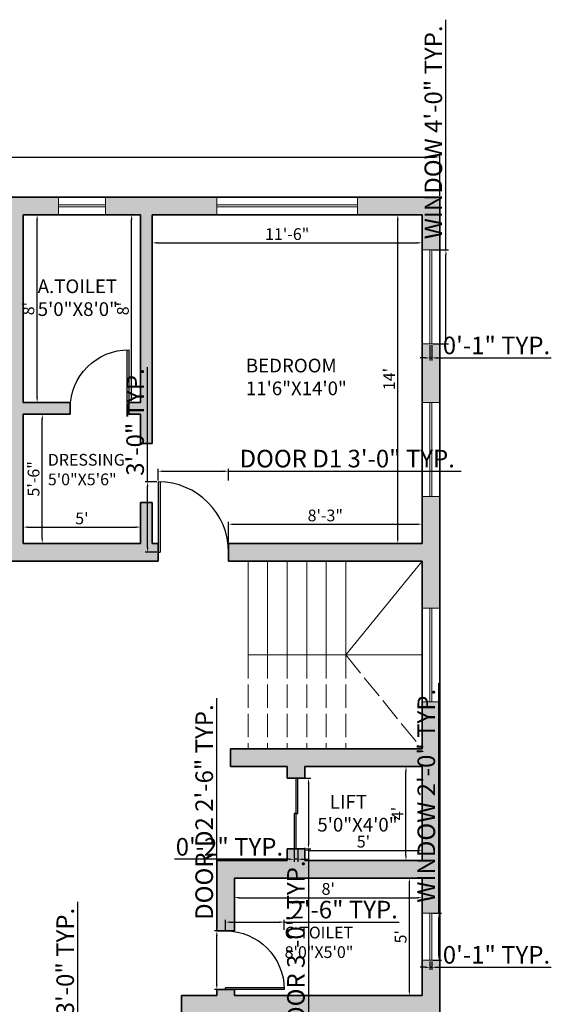
# Model space of a CAD drawing. Units: inches. Extents: x 4606 to 5879, y 1332 to 2209.
# Tile 7 of 7: x 5607 to 5879, y 1669 to 2172. Entities that reach past the tile are written whole.
import ezdxf

# ---------------------------------------------------------------- set-up
doc = ezdxf.new("R2010")
doc.units = ezdxf.units.IN
doc.linetypes.add('ACAD_ISO02W100', pattern=[15, 12, -3])
for name, color, linetype, lineweight in [('A-ANNO-DIMS', 2, 'Continuous', 18), ('A-AREA-IDEN', 7, 'Continuous', 18), ('A-DOOR', 4, 'Continuous', 25), ('A-FLOR-STRS', 7, 'Continuous', 20), ('A-FLOR-STRS-OVHD', 8, 'ACAD_ISO02W100', 13), ('A-WALL', 7, 'Continuous', 35), ('A-WALL-PATT', 252, 'Continuous', 13), ('window', 130, 'Continuous', 18)]:
    doc.layers.add(name, color=color, linetype=linetype, lineweight=lineweight)
doc.styles.get("Standard").update_dxf_attribs({"font": 'arial.ttf'})
doc.dimstyles.new('ISO-25', dxfattribs={"dimtxt": 9, "dimasz": 2.5, "dimexe": 1.25, "dimexo": 0.625, "dimtad": 1, "dimlunit": 3, "dimtxsty": 'Standard', "dimcen": 2.5, "dimadec": 0, "dimazin": 0, "dimtfac": 1, "dimtmove": 0, "dimatfit": 3, "dimfxl": 1, "dimarcsym": 0})

# ---------------------------------------------------------------- blocks, each defined once
blk = doc.blocks.new('*D25')
at = {"layer": 'A-ANNO-DIMS', "color": 0, "lineweight": -2, "transparency": 16777216}
for p, q in [((5344.86, 2081.86), (5344.86, 2102.96)), ((5347.36, 2101.71), (5819.36, 2101.71)), ((5821.86, 2081.86), (5821.86, 2102.96))]:
    blk.add_line(p, q, dxfattribs=at)
at = {"layer": 'A-ANNO-DIMS', "color": 0, "transparency": 16777216}
for points in [[(5347.36, 2102.13), (5347.36, 2101.29), (5344.86, 2101.71)], [(5819.36, 2102.13), (5819.36, 2101.29), (5821.86, 2101.71)]]:
    blk.add_solid(points, dxfattribs=at)
at = {"layer": 'Defpoints', "color": 0, "transparency": 16777216}
for p in [(5821.86, 2101.71), (5344.86, 2081.24), (5821.86, 2081.24)]:
    blk.add_point(p, dxfattribs=at)
at = {"layer": 'A-ANNO-DIMS', "color": 0, "transparency": 16777216, "insert": (5583.36, 2106.93), "char_height": 9, "attachment_point": 5}
blk.add_mtext('39\'-9"', dxfattribs=at)
blk = doc.blocks.new('D1')
for p, q in [((0, 36), (0, 0)), ((1, 36), (1, 0)), ((0, 0), (1, 0))]:
    blk.add_line(p, q)
blk.add_arc((0, 0), 36, 0, 90)
blk = doc.blocks.new('D2')
for p, q in [((0, 30), (0, 0)), ((1, 30), (1, 0)), ((0, 0), (1, 0))]:
    blk.add_line(p, q)
blk.add_arc((0, 0), 30, 0, 90)
blk = doc.blocks.new('*D29')
at = {"layer": 'A-ANNO-DIMS', "color": 0, "lineweight": -2, "transparency": 16777216}
for p, q in [((5674.86, 2071.61), (5674.86, 2056.59)), ((5812.86, 2071.61), (5812.86, 2056.59)), ((5677.36, 2057.84), (5810.36, 2057.84))]:
    blk.add_line(p, q, dxfattribs=at)
at = {"layer": 'A-ANNO-DIMS', "color": 0, "transparency": 16777216}
for points in [[(5677.36, 2058.26), (5677.36, 2057.43), (5674.86, 2057.84)], [(5810.36, 2058.26), (5810.36, 2057.43), (5812.86, 2057.84)]]:
    blk.add_solid(points, dxfattribs=at)
at = {"layer": 'Defpoints', "color": 0, "transparency": 16777216}
for p in [(5674.86, 2072.24), (5812.86, 2072.24), (5812.86, 2057.84)]:
    blk.add_point(p, dxfattribs=at)
at = {"layer": 'A-ANNO-DIMS', "color": 0, "transparency": 16777216, "insert": (5743.86, 2061.53), "char_height": 6, "attachment_point": 5}
blk.add_mtext('11\'-6"', dxfattribs=at)
blk = doc.blocks.new('*D30')
at = {"layer": 'A-ANNO-DIMS', "color": 0, "lineweight": -2, "transparency": 16777216}
for p, q in [((5812.24, 2072.24), (5799.17, 2072.24)), ((5800.42, 1906.74), (5800.42, 2069.74)), ((5812.24, 1904.24), (5799.17, 1904.24))]:
    blk.add_line(p, q, dxfattribs=at)
at = {"layer": 'A-ANNO-DIMS', "color": 0, "transparency": 16777216}
for points in [[(5800.01, 2069.74), (5800.84, 2069.74), (5800.42, 2072.24)], [(5800.01, 1906.74), (5800.84, 1906.74), (5800.42, 1904.24)]]:
    blk.add_solid(points, dxfattribs=at)
at = {"layer": 'Defpoints', "color": 0, "transparency": 16777216}
for p in [(5800.42, 2072.24), (5812.86, 2072.24), (5812.86, 1904.24)]:
    blk.add_point(p, dxfattribs=at)
at = {"layer": 'A-ANNO-DIMS', "color": 0, "transparency": 16777216, "insert": (5796.79, 1988.24), "char_height": 6, "attachment_point": 5, "rotation": 90}
blk.add_mtext("14'", dxfattribs=at)
blk = doc.blocks.new('*D33')
at = {"layer": 'A-ANNO-DIMS', "color": 0, "lineweight": -2, "transparency": 16777216}
for p, q in [((5609.49, 2072.24), (5617.21, 2072.24)), ((5615.96, 1978.74), (5615.96, 2069.74)), ((5609.49, 1976.24), (5617.21, 1976.24))]:
    blk.add_line(p, q, dxfattribs=at)
at = {"layer": 'A-ANNO-DIMS', "color": 0, "transparency": 16777216}
for points in [[(5615.54, 2069.74), (5616.37, 2069.74), (5615.96, 2072.24)], [(5615.54, 1978.74), (5616.37, 1978.74), (5615.96, 1976.24)]]:
    blk.add_solid(points, dxfattribs=at)
at = {"layer": 'Defpoints', "color": 0, "transparency": 16777216}
for p in [(5608.86, 2072.24), (5615.96, 2072.24), (5608.86, 1976.24)]:
    blk.add_point(p, dxfattribs=at)
at = {"layer": 'A-ANNO-DIMS', "color": 0, "transparency": 16777216, "insert": (5612.27, 2024.24), "char_height": 6, "attachment_point": 5, "rotation": 90}
blk.add_mtext("8'", dxfattribs=at)
blk = doc.blocks.new('*D34')
at = {"layer": 'A-ANNO-DIMS', "color": 0, "lineweight": -2, "transparency": 16777216}
for p, q in [((5668.24, 2072.24), (5663.04, 2072.24)), ((5664.29, 1978.74), (5664.29, 2069.74)), ((5668.24, 1976.24), (5663.04, 1976.24))]:
    blk.add_line(p, q, dxfattribs=at)
at = {"layer": 'A-ANNO-DIMS', "color": 0, "transparency": 16777216}
for points in [[(5663.87, 2069.74), (5664.71, 2069.74), (5664.29, 2072.24)], [(5663.87, 1978.74), (5664.71, 1978.74), (5664.29, 1976.24)]]:
    blk.add_solid(points, dxfattribs=at)
at = {"layer": 'Defpoints', "color": 0, "transparency": 16777216}
for p in [(5664.29, 2072.24), (5668.86, 2072.24), (5668.86, 1976.24)]:
    blk.add_point(p, dxfattribs=at)
at = {"layer": 'A-ANNO-DIMS', "color": 0, "transparency": 16777216, "insert": (5660.6, 2024.24), "char_height": 6, "attachment_point": 5, "rotation": 90}
blk.add_mtext("8'", dxfattribs=at)
blk = doc.blocks.new('*D39')
at = {"layer": 'A-ANNO-DIMS', "color": 0, "lineweight": -2, "transparency": 16777216}
for p, q in [((5609.49, 1970.24), (5619.83, 1970.24)), ((5618.58, 1906.74), (5618.58, 1967.74)), ((5609.49, 1904.24), (5619.83, 1904.24))]:
    blk.add_line(p, q, dxfattribs=at)
at = {"layer": 'A-ANNO-DIMS', "color": 0, "transparency": 16777216}
for points in [[(5618.17, 1967.74), (5619, 1967.74), (5618.58, 1970.24)], [(5618.17, 1906.74), (5619, 1906.74), (5618.58, 1904.24)]]:
    blk.add_solid(points, dxfattribs=at)
at = {"layer": 'Defpoints', "color": 0, "transparency": 16777216}
for p in [(5608.86, 1970.24), (5618.58, 1970.24), (5608.86, 1904.24)]:
    blk.add_point(p, dxfattribs=at)
at = {"layer": 'A-ANNO-DIMS', "color": 0, "transparency": 16777216, "insert": (5614.89, 1937.24), "char_height": 6, "attachment_point": 5, "rotation": 90}
blk.add_mtext('5\'-6"', dxfattribs=at)
blk = doc.blocks.new('*D40')
at = {"layer": 'A-ANNO-DIMS', "color": 0, "lineweight": -2, "transparency": 16777216}
for p, q in [((5608.86, 1904.86), (5608.86, 1913.83)), ((5611.36, 1912.58), (5666.36, 1912.58)), ((5668.86, 1904.86), (5668.86, 1913.83))]:
    blk.add_line(p, q, dxfattribs=at)
at = {"layer": 'A-ANNO-DIMS', "color": 0, "transparency": 16777216}
for points in [[(5611.36, 1913), (5611.36, 1912.16), (5608.86, 1912.58)], [(5666.36, 1913), (5666.36, 1912.16), (5668.86, 1912.58)]]:
    blk.add_solid(points, dxfattribs=at)
at = {"layer": 'Defpoints', "color": 0, "transparency": 16777216}
for p in [(5668.86, 1912.58), (5608.86, 1904.24), (5668.86, 1904.24)]:
    blk.add_point(p, dxfattribs=at)
at = {"layer": 'A-ANNO-DIMS', "color": 0, "transparency": 16777216, "insert": (5638.86, 1916.26), "char_height": 6, "attachment_point": 5}
blk.add_mtext("5'", dxfattribs=at)
blk = doc.blocks.new('*D41')
at = {"layer": 'A-ANNO-DIMS', "color": 0, "lineweight": -2, "transparency": 16777216}
for p, q in [((5713.86, 1904.86), (5713.86, 1915.32)), ((5716.36, 1914.07), (5810.36, 1914.07)), ((5812.86, 1904.86), (5812.86, 1915.32))]:
    blk.add_line(p, q, dxfattribs=at)
at = {"layer": 'A-ANNO-DIMS', "color": 0, "transparency": 16777216}
for points in [[(5716.36, 1914.48), (5716.36, 1913.65), (5713.86, 1914.07)], [(5810.36, 1914.48), (5810.36, 1913.65), (5812.86, 1914.07)]]:
    blk.add_solid(points, dxfattribs=at)
at = {"layer": 'Defpoints', "color": 0, "transparency": 16777216}
for p in [(5812.86, 1914.07), (5713.86, 1904.24), (5812.86, 1904.24)]:
    blk.add_point(p, dxfattribs=at)
at = {"layer": 'A-ANNO-DIMS', "color": 0, "transparency": 16777216, "insert": (5763.36, 1917.76), "char_height": 6, "attachment_point": 5}
blk.add_mtext('8\'-3"', dxfattribs=at)
blk = doc.blocks.new('*D49')
at = {"layer": 'A-ANNO-DIMS', "color": 0, "lineweight": -2, "transparency": 16777216}
for p, q in [((5812.24, 1733.24), (5805.1, 1733.24)), ((5806.35, 1675.74), (5806.35, 1730.74)), ((5812.24, 1673.24), (5805.1, 1673.24))]:
    blk.add_line(p, q, dxfattribs=at)
at = {"layer": 'A-ANNO-DIMS', "color": 0, "transparency": 16777216}
for points in [[(5805.94, 1730.74), (5806.77, 1730.74), (5806.35, 1733.24)], [(5805.94, 1675.74), (5806.77, 1675.74), (5806.35, 1673.24)]]:
    blk.add_solid(points, dxfattribs=at)
at = {"layer": 'Defpoints', "color": 0, "transparency": 16777216}
for p in [(5806.35, 1733.24), (5812.86, 1733.24), (5812.86, 1673.24)]:
    blk.add_point(p, dxfattribs=at)
at = {"layer": 'A-ANNO-DIMS', "color": 0, "transparency": 16777216, "insert": (5802.68, 1703.24), "char_height": 6, "attachment_point": 5, "rotation": 90}
blk.add_mtext("5'", dxfattribs=at)
blk = doc.blocks.new('*D50')
at = {"layer": 'A-ANNO-DIMS', "color": 0, "lineweight": -2, "transparency": 16777216}
for p, q in [((5716.86, 1732.61), (5716.86, 1721.98)), ((5812.86, 1732.61), (5812.86, 1721.98)), ((5719.36, 1723.23), (5810.36, 1723.23))]:
    blk.add_line(p, q, dxfattribs=at)
at = {"layer": 'A-ANNO-DIMS', "color": 0, "transparency": 16777216}
for points in [[(5719.36, 1723.65), (5719.36, 1722.82), (5716.86, 1723.23)], [(5810.36, 1723.65), (5810.36, 1722.82), (5812.86, 1723.23)]]:
    blk.add_solid(points, dxfattribs=at)
at = {"layer": 'Defpoints', "color": 0, "transparency": 16777216}
for p in [(5716.86, 1733.24), (5812.86, 1733.24), (5812.86, 1723.23)]:
    blk.add_point(p, dxfattribs=at)
at = {"layer": 'A-ANNO-DIMS', "color": 0, "transparency": 16777216, "insert": (5764.86, 1726.92), "char_height": 6, "attachment_point": 5}
blk.add_mtext("8'", dxfattribs=at)
blk = doc.blocks.new('*D51')
at = {"layer": 'A-ANNO-DIMS', "color": 0, "lineweight": -2, "transparency": 16777216}
for p, q in [((5752.86, 1742.86), (5752.86, 1748.66)), ((5755.36, 1747.41), (5810.36, 1747.41)), ((5812.86, 1742.86), (5812.86, 1748.66))]:
    blk.add_line(p, q, dxfattribs=at)
at = {"layer": 'A-ANNO-DIMS', "color": 0, "transparency": 16777216}
for points in [[(5755.36, 1747.82), (5755.36, 1746.99), (5752.86, 1747.41)], [(5810.36, 1747.82), (5810.36, 1746.99), (5812.86, 1747.41)]]:
    blk.add_solid(points, dxfattribs=at)
at = {"layer": 'Defpoints', "color": 0, "transparency": 16777216}
for p in [(5812.86, 1747.41), (5752.86, 1742.24), (5812.86, 1742.24)]:
    blk.add_point(p, dxfattribs=at)
at = {"layer": 'A-ANNO-DIMS', "color": 0, "transparency": 16777216, "insert": (5782.86, 1751.08), "char_height": 6, "attachment_point": 5}
blk.add_mtext("5'", dxfattribs=at)
blk = doc.blocks.new('*D52')
at = {"layer": 'A-ANNO-DIMS', "color": 0, "lineweight": -2, "transparency": 16777216}
for p, q in [((5812.24, 1790.24), (5803.37, 1790.24)), ((5804.62, 1744.74), (5804.62, 1787.74)), ((5812.24, 1742.24), (5803.37, 1742.24))]:
    blk.add_line(p, q, dxfattribs=at)
at = {"layer": 'A-ANNO-DIMS', "color": 0, "transparency": 16777216}
for points in [[(5804.21, 1787.74), (5805.04, 1787.74), (5804.62, 1790.24)], [(5804.21, 1744.74), (5805.04, 1744.74), (5804.62, 1742.24)]]:
    blk.add_solid(points, dxfattribs=at)
at = {"layer": 'Defpoints', "color": 0, "transparency": 16777216}
for p in [(5804.62, 1790.24), (5812.86, 1790.24), (5812.86, 1742.24)]:
    blk.add_point(p, dxfattribs=at)
at = {"layer": 'A-ANNO-DIMS', "color": 0, "transparency": 16777216, "insert": (5801, 1766.24), "char_height": 6, "attachment_point": 5, "rotation": 90}
blk.add_mtext("4'", dxfattribs=at)
blk = doc.blocks.new('GLAZING-72IN')
for p, q in [((0, 0), (0, 72)), ((1, 0), (1, 72))]:
    blk.add_line(p, q)
blk = doc.blocks.new('GLAZING-24IN')
for p, q in [((0, 0), (0, 24)), ((1, 0), (1, 24))]:
    blk.add_line(p, q)
blk = doc.blocks.new('GLAZING-48IN')
for p, q in [((0, 0), (0, 48)), ((1, 0), (1, 48))]:
    blk.add_line(p, q)
blk = doc.blocks.new('LIFT-DOOR-36IN')
for p, q in [((1, 0), (1, 36)), ((2, 18), (2, 36)), ((1, 18), (0, 18)), ((0, 18), (0, 0)), ((1, 18), (2, 18))]:
    blk.add_line(p, q)
blk = doc.blocks.new('*D67')
at = {"layer": 'A-ANNO-DIMS', "color": 0, "lineweight": -2, "transparency": 16777216}
for p, q in [((5825.06, 2054.24), (5825.06, 2171.88)), ((5818.49, 2054.24), (5826.31, 2054.24)), ((5825.06, 2008.74), (5825.06, 2051.74)), ((5818.49, 2006.24), (5826.31, 2006.24))]:
    blk.add_line(p, q, dxfattribs=at)
at = {"layer": 'A-ANNO-DIMS', "color": 0, "transparency": 16777216}
for points in [[(5824.65, 2051.74), (5825.48, 2051.74), (5825.06, 2054.24)], [(5824.65, 2008.74), (5825.48, 2008.74), (5825.06, 2006.24)]]:
    blk.add_solid(points, dxfattribs=at)
at = {"layer": 'Defpoints', "color": 0, "transparency": 16777216}
for p in [(5817.86, 2054.24), (5825.06, 2054.24), (5817.86, 2006.24)]:
    blk.add_point(p, dxfattribs=at)
at = {"layer": 'A-ANNO-DIMS', "color": 0, "transparency": 16777216, "insert": (5819.78, 2114.31), "char_height": 9, "attachment_point": 5, "rotation": 90}
blk.add_mtext('WINDOW 4\'-0" TYP.', dxfattribs=at)
blk = doc.blocks.new('*D68')
at = {"layer": 'A-ANNO-DIMS', "color": 0, "lineweight": -2, "transparency": 16777216}
for p, q in [((5816.86, 2005.61), (5816.86, 1997.79)), ((5817.86, 2005.61), (5817.86, 1997.79)), ((5814.36, 1999.04), (5811.86, 1999.04)), ((5816.86, 1999.04), (5817.86, 1999.04)), ((5820.36, 1999.04), (5878.97, 1999.04))]:
    blk.add_line(p, q, dxfattribs=at)
at = {"layer": 'A-ANNO-DIMS', "color": 0, "transparency": 16777216}
for points in [[(5814.36, 1999.46), (5814.36, 1998.62), (5816.86, 1999.04)], [(5820.36, 1999.46), (5820.36, 1998.62), (5817.86, 1999.04)]]:
    blk.add_solid(points, dxfattribs=at)
at = {"layer": 'Defpoints', "color": 0, "transparency": 16777216}
for p in [(5816.86, 2006.24), (5817.86, 2006.24), (5817.86, 1999.04)]:
    blk.add_point(p, dxfattribs=at)
at = {"layer": 'A-ANNO-DIMS', "color": 0, "transparency": 16777216, "insert": (5850.92, 2004.26), "char_height": 9, "attachment_point": 5}
blk.add_mtext('0\'-1" TYP.', dxfattribs=at)
blk = doc.blocks.new('*D71')
at = {"layer": 'A-ANNO-DIMS', "color": 0, "lineweight": -2, "transparency": 16777216}
for p, q in [((5821.46, 1715.24), (5821.46, 1832.88)), ((5818.49, 1715.24), (5822.71, 1715.24)), ((5821.46, 1693.74), (5821.46, 1712.74)), ((5818.49, 1691.24), (5822.71, 1691.24))]:
    blk.add_line(p, q, dxfattribs=at)
at = {"layer": 'A-ANNO-DIMS', "color": 0, "transparency": 16777216}
for points in [[(5821.05, 1712.74), (5821.88, 1712.74), (5821.46, 1715.24)], [(5821.05, 1693.74), (5821.88, 1693.74), (5821.46, 1691.24)]]:
    blk.add_solid(points, dxfattribs=at)
at = {"layer": 'Defpoints', "color": 0, "transparency": 16777216}
for p in [(5817.86, 1715.24), (5821.46, 1715.24), (5817.86, 1691.24)]:
    blk.add_point(p, dxfattribs=at)
at = {"layer": 'A-ANNO-DIMS', "color": 0, "transparency": 16777216, "insert": (5816.18, 1775.31), "char_height": 9, "attachment_point": 5, "rotation": 90}
blk.add_mtext('WINDOW 2\'-0" TYP.', dxfattribs=at)
blk = doc.blocks.new('*D72')
at = {"layer": 'A-ANNO-DIMS', "color": 0, "lineweight": -2, "transparency": 16777216}
for p, q in [((5816.86, 1690.61), (5816.86, 1686.39)), ((5817.86, 1690.61), (5817.86, 1686.39)), ((5814.36, 1687.64), (5811.86, 1687.64)), ((5816.86, 1687.64), (5817.86, 1687.64)), ((5820.36, 1687.64), (5878.97, 1687.64))]:
    blk.add_line(p, q, dxfattribs=at)
at = {"layer": 'A-ANNO-DIMS', "color": 0, "transparency": 16777216}
for points in [[(5814.36, 1688.06), (5814.36, 1687.22), (5816.86, 1687.64)], [(5820.36, 1688.06), (5820.36, 1687.22), (5817.86, 1687.64)]]:
    blk.add_solid(points, dxfattribs=at)
at = {"layer": 'Defpoints', "color": 0, "transparency": 16777216}
for p in [(5816.86, 1691.24), (5817.86, 1691.24), (5817.86, 1687.64)]:
    blk.add_point(p, dxfattribs=at)
at = {"layer": 'A-ANNO-DIMS', "color": 0, "transparency": 16777216, "insert": (5850.92, 1692.86), "char_height": 9, "attachment_point": 5}
blk.add_mtext('0\'-1" TYP.', dxfattribs=at)
blk = doc.blocks.new('*D73')
at = {"layer": 'A-ANNO-DIMS', "color": 0, "lineweight": -2, "transparency": 16777216}
for p, q in [((5707.86, 1706.24), (5707.86, 1825.18)), ((5711.74, 1706.24), (5706.61, 1706.24)), ((5707.86, 1678.74), (5707.86, 1703.74)), ((5711.74, 1676.24), (5706.61, 1676.24))]:
    blk.add_line(p, q, dxfattribs=at)
at = {"layer": 'A-ANNO-DIMS', "color": 0, "transparency": 16777216}
for points in [[(5707.45, 1703.74), (5708.28, 1703.74), (5707.86, 1706.24)], [(5707.45, 1678.74), (5708.28, 1678.74), (5707.86, 1676.24)]]:
    blk.add_solid(points, dxfattribs=at)
at = {"layer": 'Defpoints', "color": 0, "transparency": 16777216}
for p in [(5707.86, 1706.24), (5712.36, 1706.24), (5712.36, 1676.24)]:
    blk.add_point(p, dxfattribs=at)
at = {"layer": 'A-ANNO-DIMS', "color": 0, "transparency": 16777216, "insert": (5702.58, 1766.96), "char_height": 9, "attachment_point": 5, "rotation": 90}
blk.add_mtext('DOOR D2 2\'-6" TYP.', dxfattribs=at)
blk = doc.blocks.new('*D74')
at = {"layer": 'A-ANNO-DIMS', "color": 0, "lineweight": -2, "transparency": 16777216}
for p, q in [((5712.36, 1706.86), (5712.36, 1711.99)), ((5714.86, 1710.74), (5739.86, 1710.74)), ((5742.36, 1706.86), (5742.36, 1711.99)), ((5742.36, 1710.74), (5801.13, 1710.74))]:
    blk.add_line(p, q, dxfattribs=at)
at = {"layer": 'A-ANNO-DIMS', "color": 0, "transparency": 16777216}
for points in [[(5714.86, 1711.16), (5714.86, 1710.32), (5712.36, 1710.74)], [(5739.86, 1711.16), (5739.86, 1710.32), (5742.36, 1710.74)]]:
    blk.add_solid(points, dxfattribs=at)
at = {"layer": 'Defpoints', "color": 0, "transparency": 16777216}
for p in [(5742.36, 1710.74), (5712.36, 1706.24), (5742.36, 1706.24)]:
    blk.add_point(p, dxfattribs=at)
at = {"layer": 'A-ANNO-DIMS', "color": 0, "transparency": 16777216, "insert": (5773, 1715.96), "char_height": 9, "attachment_point": 5}
blk.add_mtext('2\'-6" TYP.', dxfattribs=at)
blk = doc.blocks.new('*D75')
at = {"layer": 'A-ANNO-DIMS', "color": 0, "lineweight": -2, "transparency": 16777216}
for p, q in [((5677.86, 1936.36), (5677.86, 1942.39)), ((5713.86, 1936.36), (5713.86, 1942.39)), ((5680.36, 1941.14), (5711.36, 1941.14)), ((5713.86, 1941.14), (5832.8, 1941.14))]:
    blk.add_line(p, q, dxfattribs=at)
at = {"layer": 'A-ANNO-DIMS', "color": 0, "transparency": 16777216}
for points in [[(5680.36, 1941.56), (5680.36, 1940.72), (5677.86, 1941.14)], [(5711.36, 1941.56), (5711.36, 1940.72), (5713.86, 1941.14)]]:
    blk.add_solid(points, dxfattribs=at)
at = {"layer": 'Defpoints', "color": 0, "transparency": 16777216}
for p in [(5713.86, 1941.14), (5677.86, 1935.74), (5713.86, 1935.74)]:
    blk.add_point(p, dxfattribs=at)
at = {"layer": 'A-ANNO-DIMS', "color": 0, "transparency": 16777216, "insert": (5774.58, 1946.42), "char_height": 9, "attachment_point": 5}
blk.add_mtext('DOOR D1 3\'-0" TYP.', dxfattribs=at)
blk = doc.blocks.new('*D76')
at = {"layer": 'A-ANNO-DIMS', "color": 0, "lineweight": -2, "transparency": 16777216}
for p, q in [((5672.46, 1935.74), (5672.46, 1994.34)), ((5677.24, 1935.74), (5671.21, 1935.74)), ((5672.46, 1902.24), (5672.46, 1933.24)), ((5677.24, 1899.74), (5671.21, 1899.74))]:
    blk.add_line(p, q, dxfattribs=at)
at = {"layer": 'A-ANNO-DIMS', "color": 0, "transparency": 16777216}
for points in [[(5672.05, 1933.24), (5672.88, 1933.24), (5672.46, 1935.74)], [(5672.05, 1902.24), (5672.88, 1902.24), (5672.46, 1899.74)]]:
    blk.add_solid(points, dxfattribs=at)
at = {"layer": 'Defpoints', "color": 0, "transparency": 16777216}
for p in [(5672.46, 1935.74), (5677.86, 1935.74), (5677.86, 1899.74)]:
    blk.add_point(p, dxfattribs=at)
at = {"layer": 'A-ANNO-DIMS', "color": 0, "transparency": 16777216, "insert": (5667.24, 1966.29), "char_height": 9, "attachment_point": 5, "rotation": 90}
blk.add_mtext('3\'-0" TYP.', dxfattribs=at)
blk = doc.blocks.new('*D79')
at = {"layer": 'A-ANNO-DIMS', "color": 0, "lineweight": -2, "transparency": 16777216}
for p, q in [((5636.76, 1602.24), (5636.76, 1721.18)), ((5631.99, 1602.24), (5638.01, 1602.24)), ((5636.76, 1568.74), (5636.76, 1599.74)), ((5631.99, 1566.24), (5638.01, 1566.24))]:
    blk.add_line(p, q, dxfattribs=at)
at = {"layer": 'A-ANNO-DIMS', "color": 0, "transparency": 16777216}
for points in [[(5636.35, 1599.74), (5637.18, 1599.74), (5636.76, 1602.24)], [(5636.35, 1568.74), (5637.18, 1568.74), (5636.76, 1566.24)]]:
    blk.add_solid(points, dxfattribs=at)
at = {"layer": 'Defpoints', "color": 0, "transparency": 16777216}
for p in [(5631.36, 1602.24), (5636.76, 1602.24), (5631.36, 1566.24)]:
    blk.add_point(p, dxfattribs=at)
at = {"layer": 'A-ANNO-DIMS', "color": 0, "transparency": 16777216, "insert": (5631.48, 1662.96), "char_height": 9, "attachment_point": 5, "rotation": 90}
blk.add_mtext('DOOR D3 3\'-0" TYP.', dxfattribs=at)
blk = doc.blocks.new('*D81')
at = {"layer": 'A-ANNO-DIMS', "color": 0, "lineweight": -2, "transparency": 16777216}
for p, q in [((5749.99, 1784.24), (5756.01, 1784.24)), ((5754.76, 1781.74), (5754.76, 1750.74)), ((5749.99, 1748.24), (5756.01, 1748.24)), ((5754.76, 1748.24), (5754.76, 1619.48))]:
    blk.add_line(p, q, dxfattribs=at)
at = {"layer": 'A-ANNO-DIMS', "color": 0, "transparency": 16777216}
for points in [[(5754.35, 1781.74), (5755.18, 1781.74), (5754.76, 1784.24)], [(5754.35, 1750.74), (5755.18, 1750.74), (5754.76, 1748.24)]]:
    blk.add_solid(points, dxfattribs=at)
at = {"layer": 'Defpoints', "color": 0, "transparency": 16777216}
for p in [(5749.36, 1784.24), (5749.36, 1748.24), (5754.76, 1748.24)]:
    blk.add_point(p, dxfattribs=at)
at = {"layer": 'A-ANNO-DIMS', "color": 0, "transparency": 16777216, "insert": (5749.48, 1682.61), "char_height": 9, "attachment_point": 5, "rotation": 90}
blk.add_mtext('LIFT DOOR 3\'-0" TYP.', dxfattribs=at)
blk = doc.blocks.new('*D82')
at = {"layer": 'A-ANNO-DIMS', "color": 0, "lineweight": -2, "transparency": 16777216}
for p, q in [((5747.36, 1747.61), (5747.36, 1741.59)), ((5749.36, 1747.61), (5749.36, 1741.59)), ((5744.86, 1742.84), (5686.25, 1742.84)), ((5749.36, 1742.84), (5747.36, 1742.84)), ((5751.86, 1742.84), (5754.36, 1742.84))]:
    blk.add_line(p, q, dxfattribs=at)
at = {"layer": 'A-ANNO-DIMS', "color": 0, "transparency": 16777216}
for points in [[(5744.86, 1743.26), (5744.86, 1742.42), (5747.36, 1742.84)], [(5751.86, 1743.26), (5751.86, 1742.42), (5749.36, 1742.84)]]:
    blk.add_solid(points, dxfattribs=at)
at = {"layer": 'Defpoints', "color": 0, "transparency": 16777216}
for p in [(5747.36, 1748.24), (5749.36, 1748.24), (5747.36, 1742.84)]:
    blk.add_point(p, dxfattribs=at)
at = {"layer": 'A-ANNO-DIMS', "color": 0, "transparency": 16777216, "insert": (5714.31, 1748.06), "char_height": 9, "attachment_point": 5}
blk.add_mtext('0\'-2" TYP.', dxfattribs=at)

msp = doc.modelspace()

# ---------------------------------------------------------------- hatches: boundary and pattern name
at = {"layer": 'A-WALL-PATT', "transparency": 33554687}
h = msp.add_hatch(color=256, dxfattribs=at)
h.dxf.hatch_style = 1
h.paths.add_polyline_path([(5635.864, 1512.239), (5626.864, 1512.239), (5626.864, 1420.239), (5566.864, 1420.239), (5566.864, 1545.239), (5626.864, 1545.239), (5626.864, 1542.239), (5631.364, 1542.239), (5635.864, 1542.239), (5635.864, 1566.239), (5626.864, 1566.239), (5626.864, 1554.239), (5566.864, 1554.239), (5566.864, 1614.239), (5626.864, 1614.239), (5626.864, 1602.239), (5631.364, 1602.239), (5635.864, 1602.239), (5635.864, 1623.239), (5512.864, 1623.239), (5512.864, 1614.239), (5557.864, 1614.239), (5557.864, 1554.239), (5512.864, 1554.239), (5512.864, 1549.739), (5512.864, 1545.239), (5557.864, 1545.239), (5557.864, 1411.239), (5683.864, 1411.239), (5683.864, 1420.239), (5635.864, 1420.239)])
h.paths.add_polyline_path([(5788.864, 1446.239), (5779.864, 1446.239), (5779.864, 1420.239), (5731.864, 1420.239), (5731.864, 1411.239), (5788.864, 1411.239)])
h.paths.add_polyline_path([(5788.864, 1512.239), (5779.864, 1512.239), (5779.864, 1494.239), (5788.864, 1494.239)])
h.paths.add_polyline_path([(5788.864, 1591.739), (5779.864, 1591.739), (5779.864, 1542.239), (5788.864, 1542.239)])
h.paths.add_polyline_path([(5821.864, 1691.239), (5812.864, 1691.239), (5812.864, 1673.239), (5716.864, 1673.239), (5716.864, 1676.239), (5712.364, 1676.239), (5707.864, 1676.239), (5707.864, 1673.239), (5689.864, 1673.239), (5689.864, 1664.239), (5779.864, 1664.239), (5779.864, 1639.739), (5788.864, 1639.739), (5788.864, 1664.239), (5821.864, 1664.239)])
h.paths.add_polyline_path([(5821.864, 1823.239), (5812.864, 1823.239), (5812.864, 1799.239), (5714.864, 1799.239), (5714.864, 1790.239), (5743.864, 1790.239), (5743.864, 1784.239), (5752.864, 1784.239), (5752.864, 1790.239), (5812.864, 1790.239), (5812.864, 1742.239), (5752.864, 1742.239), (5752.864, 1748.239), (5743.864, 1748.239), (5743.864, 1742.239), (5707.864, 1742.239), (5707.864, 1706.239), (5716.864, 1706.239), (5716.864, 1733.239), (5812.864, 1733.239), (5812.864, 1715.239), (5821.864, 1715.239)])
h.paths.add_polyline_path([(5821.864, 1928.239), (5812.864, 1928.239), (5812.864, 1904.239), (5713.864, 1904.239), (5713.864, 1895.239), (5812.864, 1895.239), (5812.864, 1871.239), (5821.864, 1871.239)])
h.paths.add_polyline_path([(5821.864, 2006.239), (5812.864, 2006.239), (5812.864, 1976.239), (5821.864, 1976.239)])
h.paths.add_polyline_path([(5821.864, 2081.239), (5779.864, 2081.239), (5779.864, 2072.239), (5812.864, 2072.239), (5812.864, 2054.239), (5821.864, 2054.239)])
h.paths.add_polyline_path([(5707.864, 2081.239), (5650.864, 2081.239), (5650.864, 2072.239), (5668.864, 2072.239), (5668.864, 1976.239), (5662.864, 1976.239), (5662.864, 1970.239), (5668.864, 1970.239), (5668.864, 1955.239), (5674.864, 1955.239), (5674.864, 2072.239), (5707.864, 2072.239)])
h.paths.add_polyline_path([(5626.864, 2081.239), (5578.864, 2081.239), (5578.864, 2072.239), (5602.864, 2072.239), (5602.864, 1976.239), (5566.864, 1976.239), (5566.864, 1970.239), (5602.864, 1970.239), (5602.864, 1904.239), (5530.864, 1904.239), (5530.864, 1925.239), (5521.864, 1925.239), (5521.864, 1904.239), (5518.864, 1904.239), (5518.864, 1895.239), (5605.864, 1895.239), (5677.864, 1895.239), (5677.864, 1904.239), (5674.864, 1904.239), (5674.864, 1925.239), (5668.864, 1925.239), (5668.864, 1904.239), (5608.864, 1904.239), (5608.864, 1970.239), (5632.864, 1970.239), (5632.864, 1976.239), (5608.864, 1976.239), (5608.864, 2072.239), (5626.864, 2072.239)])
h.paths.add_polyline_path([(5554.864, 2081.239), (5473.864, 2081.239), (5473.864, 2072.239), (5521.864, 2072.239), (5521.864, 1955.239), (5530.864, 1955.239), (5530.864, 1970.239), (5536.864, 1970.239), (5536.864, 1976.239), (5530.864, 1976.239), (5530.864, 2072.239), (5554.864, 2072.239)])
h.paths.add_polyline_path([(5401.864, 2081.239), (5344.864, 2081.239), (5344.864, 2054.239), (5353.864, 2054.239), (5353.864, 2072.239), (5401.864, 2072.239)])
h.paths.add_polyline_path([(5353.864, 2006.239), (5344.864, 2006.239), (5344.864, 1970.239), (5353.864, 1970.239)])
h.paths.add_polyline_path([(5482.864, 1904.239), (5353.864, 1904.239), (5353.864, 1922.239), (5344.864, 1922.239), (5344.864, 1895.239), (5452.864, 1895.239), (5452.864, 1674.239), (5461.864, 1674.239), (5461.864, 1895.239), (5482.864, 1895.239)])
h.paths.add_polyline_path([(5461.864, 1602.239), (5452.864, 1602.239), (5452.864, 1474.239), (5461.864, 1474.239), (5461.864, 1545.239), (5464.864, 1545.239), (5464.864, 1554.239), (5461.864, 1554.239)])

# ---------------------------------------------------------------- linework, layer by layer
at = {"layer": 'A-FLOR-STRS'}
for p, q in [((5723.864, 1847.239), (5723.864, 1895.239)), ((5733.864, 1847.239), (5733.864, 1895.239)), ((5743.864, 1847.239), (5743.864, 1895.239)), ((5753.864, 1847.239), (5753.864, 1895.239)), ((5763.864, 1847.239), (5763.864, 1895.239)), ((5773.864, 1847.239), (5773.864, 1895.239)), ((5773.864, 1847.239), (5812.864, 1895.239)), ((5723.864, 1847.239), (5812.864, 1847.239))]:
    msp.add_line(p, q, dxfattribs=at)
at = {"layer": 'A-FLOR-STRS-OVHD'}
for p, q in [((5723.864, 1847.239), (5723.864, 1799.239)), ((5733.864, 1847.239), (5733.864, 1799.239)), ((5743.864, 1847.239), (5743.864, 1799.239)), ((5753.864, 1847.239), (5753.864, 1799.239)), ((5763.864, 1847.239), (5763.864, 1799.239)), ((5773.864, 1847.239), (5773.864, 1799.239)), ((5773.864, 1847.239), (5812.864, 1799.239))]:
    msp.add_line(p, q, dxfattribs=at)
at = {"layer": 'A-WALL'}
for p, q in [((5668.864, 2072.239), (5608.864, 2072.239)), ((5608.864, 2072.239), (5608.864, 1976.239)), ((5668.864, 2072.239), (5668.864, 1976.239)), ((5812.864, 2072.239), (5674.864, 2072.239)), ((5674.864, 2072.239), (5674.864, 1955.239)), ((5812.864, 1904.239), (5812.864, 2072.239)), ((5632.864, 1976.239), (5608.864, 1976.239)), ((5632.864, 1976.239), (5632.864, 1970.239)), ((5668.864, 1976.239), (5662.864, 1976.239)), ((5662.864, 1976.239), (5662.864, 1970.239)), ((5632.864, 1970.239), (5608.864, 1970.239)), ((5608.864, 1970.239), (5608.864, 1904.239)), ((5668.864, 1970.239), (5662.864, 1970.239)), ((5668.864, 1970.239), (5668.864, 1955.239)), ((5674.864, 1955.239), (5668.864, 1955.239)), ((5674.864, 1925.239), (5668.864, 1925.239)), ((5668.864, 1925.239), (5668.864, 1904.239)), ((5674.864, 1925.239), (5674.864, 1904.239)), ((5668.864, 1904.239), (5608.864, 1904.239)), ((5677.864, 1904.239), (5674.864, 1904.239)), ((5677.864, 1904.239), (5677.864, 1895.239)), ((5812.864, 1904.239), (5713.864, 1904.239)), ((5713.864, 1904.239), (5713.864, 1895.239)), ((5677.864, 1895.239), (5518.864, 1895.239)), ((5812.864, 1895.239), (5713.864, 1895.239)), ((5812.864, 1799.239), (5812.864, 1895.239)), ((5812.864, 1799.239), (5714.864, 1799.239)), ((5714.864, 1799.239), (5714.864, 1790.239)), ((5743.864, 1790.239), (5714.864, 1790.239)), ((5743.864, 1784.239), (5743.864, 1790.239)), ((5812.864, 1790.239), (5752.864, 1790.239)), ((5752.864, 1784.239), (5752.864, 1790.239)), ((5812.864, 1742.239), (5812.864, 1790.239)), ((5752.864, 1784.239), (5743.864, 1784.239)), ((5752.864, 1748.239), (5743.864, 1748.239)), ((5743.864, 1742.239), (5743.864, 1748.239)), ((5752.864, 1742.239), (5752.864, 1748.239)), ((5743.864, 1742.239), (5707.864, 1742.239)), ((5707.864, 1706.239), (5707.864, 1742.239)), ((5812.864, 1742.239), (5752.864, 1742.239)), ((5812.864, 1733.239), (5716.864, 1733.239)), ((5716.864, 1706.239), (5716.864, 1733.239)), ((5812.864, 1673.239), (5812.864, 1733.239)), ((5716.864, 1706.239), (5707.864, 1706.239)), ((5716.864, 1676.239), (5707.864, 1676.239)), ((5707.864, 1673.239), (5707.864, 1676.239)), ((5716.864, 1673.239), (5716.864, 1676.239)), ((5707.864, 1673.239), (5689.864, 1673.239)), ((5689.864, 1664.239), (5689.864, 1673.239)), ((5812.864, 1673.239), (5716.864, 1673.239))]:
    msp.add_line(p, q, dxfattribs=at)
msp.add_lwpolyline([(5821.864, 1664.239), (5821.864, 2081.239), (5344.864, 2081.239), (5344.864, 1411.239), (5788.864, 1411.239)], dxfattribs=at)
at = {"layer": 'window'}
for p, q in [((5626.864, 2072.239), (5626.864, 2081.239)), ((5650.864, 2072.239), (5650.864, 2081.239)), ((5707.864, 2072.239), (5707.864, 2081.239)), ((5779.864, 2072.239), (5779.864, 2081.239)), ((5821.864, 2054.239), (5812.864, 2054.239)), ((5821.864, 2006.239), (5812.864, 2006.239)), ((5821.864, 1976.239), (5812.864, 1976.239)), ((5821.864, 1928.239), (5812.864, 1928.239)), ((5812.864, 1871.239), (5821.864, 1871.239)), ((5812.864, 1823.239), (5821.864, 1823.239)), ((5812.864, 1715.239), (5821.864, 1715.239)), ((5812.864, 1691.239), (5821.864, 1691.239))]:
    msp.add_line(p, q, dxfattribs=at)

# ---------------------------------------------------------------- block references
at = {"layer": 'A-DOOR', "xscale": -1}
msp.add_blockref('D2', (5662.864, 1973.239), dxfattribs=at)
at = {"layer": 'A-DOOR'}
msp.add_blockref('D1', (5677.864, 1899.739), dxfattribs=at)
at = {"layer": 'A-DOOR', "rotation": 180}
msp.add_blockref('LIFT-DOOR-36IN', (5749.364, 1784.239), dxfattribs=at)
at = {"layer": 'A-DOOR', "xscale": -1, "rotation": 270}
msp.add_blockref('D2', (5712.364, 1676.239), dxfattribs=at)
at = {"layer": 'window'}
for name, p, rotation in [('GLAZING-24IN', (5650.864, 2076.239), 89.99999999999984), ('GLAZING-72IN', (5779.864, 2076.239), 90.00000000000003)]:
    msp.add_blockref(name, p, dxfattribs=dict(at, rotation=rotation))
for name, p in [('GLAZING-48IN', (5816.864, 2006.239)), ('GLAZING-48IN', (5816.864, 1928.239)), ('GLAZING-48IN', (5816.864, 1823.239)), ('GLAZING-24IN', (5816.864, 1691.239))]:
    msp.add_blockref(name, p, dxfattribs=at)

# ---------------------------------------------------------------- texts
at = {"layer": 'A-AREA-IDEN', "attachment_point": 1}
for s, insert, char_height in [('{\\fTimes New Roman|b0|i0|c0|p18;A.TOILET\\P5\'0"X8\'0"}', (5616.251, 2039.149), 7), ('{\\fTimes New Roman|b0|i0|c0|p18;BEDROOM\\P11\'6"X14\'0"}', (5722.728, 1998.647), 7), ('{\\fTimes New Roman|b0|i0|c0|p18;DRESSING\\P5\'0"X5\'6"}', (5621.43, 1949.974), 6), ('{\\fTimes New Roman|b0|i0|c0|p18;   LIFT\\P5\'0"X4\'0"}', (5759.289, 1775.694), 7), ('{\\fTimes New Roman|b0|i0|c0|p18;C.TOILET\\P8\'0"X5\'0"}', (5742.546, 1708.408), 6)]:
    msp.add_mtext_dynamic_manual_height_columns(s, width=80.30411, gutter_width=12.5, heights=[0], dxfattribs=dict(at, insert=insert, char_height=char_height))

# ---------------------------------------------------------------- dimensions: what is measured, and where the dimension line sits
at = {"layer": 'A-ANNO-DIMS'}
for base, p1, p2, angle, text, picture, middle in [((5825.064, 2054.239), (5817.864, 2006.239), (5817.864, 2054.239), 90, 'WINDOW <> TYP.', '*D67', (5819.783, 2114.308)), ((5672.464, 1935.739), (5677.864, 1899.739), (5677.864, 1935.739), 90, '<> TYP.', '*D76', (5667.241, 1966.291)), ((5821.464, 1715.239), (5817.864, 1691.239), (5817.864, 1715.239), 90, 'WINDOW <> TYP.', '*D71', (5816.183, 1775.308)), ((5707.864, 1706.239), (5712.364, 1676.239), (5712.364, 1706.239), 90, 'DOOR D2 <> TYP.', '*D73', (5702.583, 1766.958)), ((5754.764, 1748.239), (5749.364, 1784.239), (5749.364, 1748.239), 270, 'LIFT DOOR <> TYP.', '*D81', (5749.48, 1682.608)), ((5747.364, 1742.839), (5749.364, 1748.239), (5747.364, 1748.239), 180, '<> TYP.', '*D82', (5714.31, 1748.059)), ((5636.764, 1602.239), (5631.364, 1566.239), (5631.364, 1602.239), 90, 'DOOR D3 <> TYP.', '*D79', (5631.48, 1662.958))]:
    dim = msp.add_linear_dim(base=base, p1=p1, p2=p2, angle=angle, text=text, dimstyle='ISO-25', override={"dimdec": 1, "dimlfac": 1, "dimrnd": 0, "dimzin": 1, "dimdsep": 46, "dimlunit": 4, "dimfrac": 2}, dxfattribs=at)
    dim.commit()
    dim.dimension.update_dxf_attribs({"geometry": picture, "text_midpoint": middle})
for base, p1, p2, override, picture, middle in [((5821.864, 2101.71), (5344.864, 2081.239), (5821.864, 2081.239), {"dimclrd": 0, "dimclre": 0, "dimclrt": 0}, '*D25', (5583.364, 2106.933)), ((5812.864, 2057.845), (5674.864, 2072.239), (5812.864, 2072.239), {"dimtxt": 6, "dimclrd": 0, "dimclre": 0, "dimclrt": 0}, '*D29', (5743.864, 2061.533)), ((5668.864, 1912.582), (5608.864, 1904.239), (5668.864, 1904.239), {"dimtxt": 6, "dimclrd": 0, "dimclre": 0, "dimclrt": 0}, '*D40', (5638.864, 1916.258)), ((5812.864, 1914.067), (5713.864, 1904.239), (5812.864, 1904.239), {"dimtxt": 6, "dimclrd": 0, "dimclre": 0, "dimclrt": 0}, '*D41', (5763.364, 1917.757)), ((5812.864, 1747.408), (5752.864, 1742.239), (5812.864, 1742.239), {"dimtxt": 6, "dimclrd": 0, "dimclre": 0, "dimclrt": 0}, '*D51', (5782.864, 1751.084)), ((5812.864, 1723.234), (5716.864, 1733.239), (5812.864, 1733.239), {"dimtxt": 6, "dimclrd": 0, "dimclre": 0, "dimclrt": 0}, '*D50', (5764.864, 1726.922))]:
    dim = msp.add_linear_dim(base=base, p1=p1, p2=p2, dimstyle='ISO-25', override=override, dxfattribs=at)
    dim.commit()
    dim.dimension.update_dxf_attribs({"geometry": picture, "text_midpoint": middle})
for base, p1, p2, picture, middle in [((5615.958, 2072.239), (5608.864, 1976.239), (5608.864, 2072.239), '*D33', (5612.27, 2024.239)), ((5664.29, 2072.239), (5668.864, 1976.239), (5668.864, 2072.239), '*D34', (5660.602, 2024.239)), ((5800.422, 2072.239), (5812.864, 1904.239), (5812.864, 2072.239), '*D30', (5796.785, 1988.239)), ((5618.582, 1970.239), (5608.864, 1904.239), (5608.864, 1970.239), '*D39', (5614.893, 1937.239)), ((5804.622, 1790.239), (5812.864, 1742.239), (5812.864, 1790.239), '*D52', (5800.997, 1766.239)), ((5806.353, 1733.239), (5812.864, 1673.239), (5812.864, 1733.239), '*D49', (5802.677, 1703.239))]:
    dim = msp.add_linear_dim(base=base, p1=p1, p2=p2, angle=270, dimstyle='ISO-25', override={"dimtxt": 6, "dimclrd": 0, "dimclre": 0, "dimclrt": 0}, dxfattribs=at)
    dim.commit()
    dim.dimension.update_dxf_attribs({"geometry": picture, "text_midpoint": middle})
for base, p1, p2, text, picture, middle in [((5817.864, 1999.039), (5816.864, 2006.239), (5817.864, 2006.239), '<> TYP.', '*D68', (5850.919, 2004.259)), ((5713.864, 1941.139), (5677.864, 1935.739), (5713.864, 1935.739), 'DOOR D1 <> TYP.', '*D75', (5774.584, 1946.424)), ((5742.364, 1710.739), (5712.364, 1706.239), (5742.364, 1706.239), '<> TYP.', '*D74', (5772.996, 1715.959)), ((5817.864, 1687.639), (5816.864, 1691.239), (5817.864, 1691.239), '<> TYP.', '*D72', (5850.919, 1692.859))]:
    dim = msp.add_linear_dim(base=base, p1=p1, p2=p2, text=text, dimstyle='ISO-25', override={"dimdec": 1, "dimlfac": 1, "dimrnd": 0, "dimzin": 1, "dimdsep": 46, "dimlunit": 4, "dimfrac": 2}, dxfattribs=at)
    dim.commit()
    dim.dimension.update_dxf_attribs({"geometry": picture, "text_midpoint": middle})

doc.saveas('drawing.dxf')
